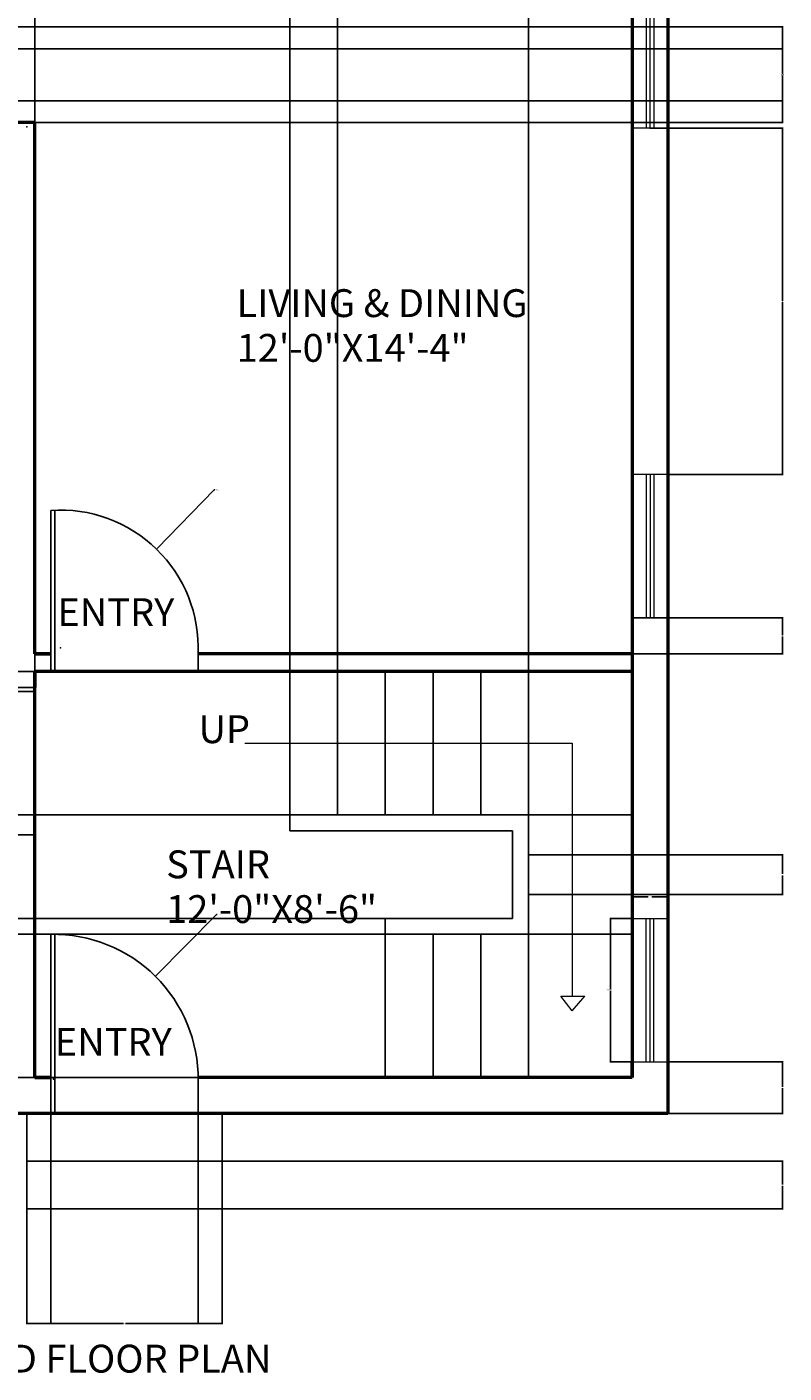
# Model space of a CAD drawing. Units: inches. Extents: x 2750 to 3097, y 1429 to 2028.
# Tile 2 of 4: x 2907 to 3097, y 1429 to 1768. Entities that reach past the tile are written whole.
import ezdxf

# ---------------------------------------------------------------- set-up
doc = ezdxf.new("R2010")
doc.units = ezdxf.units.IN
for name, color, linetype, lineweight in [('A-ANNO-DIMS', 2, 'Continuous', 18), ('A-ANNO-SYMB', 7, 'Continuous', 18), ('A-ANNO-TEXT', 7, 'Continuous', 25), ('A-AREA-IDEN', 7, 'Continuous', 25), ('A-DOOR', 3, 'Continuous', 25), ('A-FLOR-STRS', 7, 'Continuous', 25), ('A-GLAZ', 4, 'Continuous', 18), ('A-WALL', 7, 'Continuous', 50)]:
    doc.layers.add(name, color=color, linetype=linetype, lineweight=lineweight)
doc.styles.get("Standard").update_dxf_attribs({"font": 'arial.ttf'})
doc.dimstyles.get("Standard").update_dxf_attribs({"dimtxt": 0.18, "dimasz": 0.18, "dimexe": 0.18, "dimexo": 0.0625, "dimgap": 0.09, "dimtad": 0, "dimtih": 1, "dimtoh": 1, "dimdec": 4, "dimzin": 0, "dimdsep": 46, "dimtxsty": 'Standard', "dimcen": 0.09, "dimadec": 0, "dimazin": 0, "dimtfac": 1, "dimtdec": 4, "dimtofl": 0, "dimtmove": 0, "dimatfit": 3, "dimfxl": 1, "dimtolj": 1, "dimtzin": 0, "dimarcsym": 0})

# ---------------------------------------------------------------- blocks, each defined once
blk = doc.blocks.new('WIN-36IN')
for p, q in [((9, 36), (0, 36)), ((3.5, 36), (3.5, 0)), ((4.5, 36), (4.5, 0)), ((5.5, 36), (5.5, 0)), ((9, 0), (0, 0))]:
    blk.add_line(p, q)
blk = doc.blocks.new('*D7')
at = {"layer": 'A-ANNO-DIMS', "color": 0, "lineweight": -2, "transparency": 16777216}
for p, q in [((3058.46, 1543.59), (3052.94, 1543.59)), ((3053.12, 1543.41), (3053.12, 1525.78)), ((3053.12, 1507.77), (3053.12, 1525.41)), ((3058.46, 1507.59), (3052.94, 1507.59))]:
    blk.add_line(p, q, dxfattribs=at)
at = {"layer": 'A-ANNO-DIMS', "color": 0, "transparency": 16777216}
for points in [[(3053.09, 1543.41), (3053.15, 1543.41), (3053.12, 1543.59)], [(3053.09, 1507.77), (3053.15, 1507.77), (3053.12, 1507.59)]]:
    blk.add_solid(points, dxfattribs=at)
at = {"layer": 'Defpoints', "color": 0, "transparency": 16777216}
for p in [(3058.52, 1543.59), (3053.12, 1507.59), (3058.52, 1507.59)]:
    blk.add_point(p, dxfattribs=at)
at = {"layer": 'A-ANNO-DIMS', "color": 0, "transparency": 16777216, "insert": (3053.12, 1525.59), "char_height": 0.18, "attachment_point": 5}
blk.add_mtext('\\A1;WINDOW 36 TYP.', dxfattribs=at)
blk = doc.blocks.new('*D8')
at = {"layer": 'A-ANNO-DIMS', "color": 0, "lineweight": -2, "transparency": 16777216}
for p, q in [((3058.52, 1543.66), (3058.52, 1549.17)), ((3058.7, 1548.99), (3062.56, 1548.99)), ((3067.34, 1548.99), (3063.48, 1548.99)), ((3067.52, 1543.66), (3067.52, 1549.17))]:
    blk.add_line(p, q, dxfattribs=at)
at = {"layer": 'A-ANNO-DIMS', "color": 0, "transparency": 16777216}
for points in [[(3058.7, 1549.02), (3058.7, 1548.96), (3058.52, 1548.99)], [(3067.34, 1549.02), (3067.34, 1548.96), (3067.52, 1548.99)]]:
    blk.add_solid(points, dxfattribs=at)
at = {"layer": 'Defpoints', "color": 0, "transparency": 16777216}
for p in [(3058.52, 1548.99), (3058.52, 1543.59), (3067.52, 1543.59)]:
    blk.add_point(p, dxfattribs=at)
at = {"layer": 'A-ANNO-DIMS', "color": 0, "transparency": 16777216, "insert": (3063.02, 1548.99), "char_height": 0.18, "attachment_point": 5}
blk.add_mtext('\\A1;9 TYP.', dxfattribs=at)
blk = doc.blocks.new('*D16')
at = {"layer": 'A-ANNO-DIMS', "color": 0, "lineweight": -2, "transparency": 16777216}
for p, q in [((2906.52, 1470.53), (2906.52, 1441.61)), ((2955.52, 1470.53), (2955.52, 1441.61)), ((2906.7, 1441.79), (2930.8, 1441.79)), ((2955.34, 1441.79), (2931.24, 1441.79))]:
    blk.add_line(p, q, dxfattribs=at)
at = {"layer": 'A-ANNO-DIMS', "color": 0, "transparency": 16777216}
for points in [[(2906.7, 1441.82), (2906.7, 1441.76), (2906.52, 1441.79)], [(2955.34, 1441.82), (2955.34, 1441.76), (2955.52, 1441.79)]]:
    blk.add_solid(points, dxfattribs=at)
at = {"layer": 'Defpoints', "color": 0, "transparency": 16777216}
for p in [(2906.52, 1470.59), (2955.52, 1470.59), (2955.52, 1441.79)]:
    blk.add_point(p, dxfattribs=at)
at = {"layer": 'A-ANNO-DIMS', "color": 0, "transparency": 16777216, "insert": (2931.02, 1441.79), "char_height": 0.18, "attachment_point": 5}
blk.add_mtext('\\A1;49', dxfattribs=at)
blk = doc.blocks.new('*D19')
at = {"layer": 'A-ANNO-DIMS', "color": 0, "lineweight": -2, "transparency": 16777216}
for p, q in [((2912.52, 1494.53), (2912.52, 1441.61)), ((2949.52, 1494.53), (2949.52, 1441.61)), ((2912.7, 1441.79), (2930.8, 1441.79)), ((2949.34, 1441.79), (2931.24, 1441.79))]:
    blk.add_line(p, q, dxfattribs=at)
at = {"layer": 'A-ANNO-DIMS', "color": 0, "transparency": 16777216}
for points in [[(2912.7, 1441.82), (2912.7, 1441.76), (2912.52, 1441.79)], [(2949.34, 1441.82), (2949.34, 1441.76), (2949.52, 1441.79)]]:
    blk.add_solid(points, dxfattribs=at)
at = {"layer": 'Defpoints', "color": 0, "transparency": 16777216}
for p in [(2912.52, 1494.59), (2949.52, 1494.59), (2949.52, 1441.79)]:
    blk.add_point(p, dxfattribs=at)
at = {"layer": 'A-ANNO-DIMS', "color": 0, "transparency": 16777216, "insert": (2931.02, 1441.79), "char_height": 0.18, "attachment_point": 5}
blk.add_mtext('\\A1;37', dxfattribs=at)
blk = doc.blocks.new('*D24')
at = {"layer": 'A-ANNO-DIMS', "color": 0, "lineweight": -2, "transparency": 16777216}
for p, q in [((3067.58, 1507.59), (3096.5, 1507.59)), ((3096.32, 1507.41), (3096.32, 1501.27)), ((3096.32, 1494.77), (3096.32, 1500.91)), ((3067.58, 1494.59), (3096.5, 1494.59))]:
    blk.add_line(p, q, dxfattribs=at)
at = {"layer": 'A-ANNO-DIMS', "color": 0, "transparency": 16777216}
for points in [[(3096.29, 1507.41), (3096.35, 1507.41), (3096.32, 1507.59)], [(3096.29, 1494.77), (3096.35, 1494.77), (3096.32, 1494.59)]]:
    blk.add_solid(points, dxfattribs=at)
at = {"layer": 'Defpoints', "color": 0, "transparency": 16777216}
for p in [(3067.52, 1507.59), (3096.32, 1507.59), (3067.52, 1494.59)]:
    blk.add_point(p, dxfattribs=at)
at = {"layer": 'A-ANNO-DIMS', "color": 0, "transparency": 16777216, "insert": (3096.32, 1501.09), "char_height": 0.18, "attachment_point": 5}
blk.add_mtext('\\A1;13', dxfattribs=at)
blk = doc.blocks.new('*D25')
at = {"layer": 'A-ANNO-DIMS', "color": 0, "lineweight": -2, "transparency": 16777216}
for p, q in [((3058.58, 1619.09), (3096.5, 1619.09)), ((3096.32, 1618.91), (3096.32, 1614.77)), ((3096.32, 1610.27), (3096.32, 1614.41)), ((3058.58, 1610.09), (3096.5, 1610.09))]:
    blk.add_line(p, q, dxfattribs=at)
at = {"layer": 'A-ANNO-DIMS', "color": 0, "transparency": 16777216}
for points in [[(3096.29, 1618.91), (3096.35, 1618.91), (3096.32, 1619.09)], [(3096.29, 1610.27), (3096.35, 1610.27), (3096.32, 1610.09)]]:
    blk.add_solid(points, dxfattribs=at)
at = {"layer": 'Defpoints', "color": 0, "transparency": 16777216}
for p in [(3058.52, 1619.09), (3096.32, 1619.09), (3058.52, 1610.09)]:
    blk.add_point(p, dxfattribs=at)
at = {"layer": 'A-ANNO-DIMS', "color": 0, "transparency": 16777216, "insert": (3096.32, 1614.59), "char_height": 0.18, "attachment_point": 5}
blk.add_mtext('\\A1;9', dxfattribs=at)
blk = doc.blocks.new('*D26')
at = {"layer": 'A-ANNO-DIMS', "color": 0, "lineweight": -2, "transparency": 16777216}
for p, q in [((3067.58, 1742.09), (3096.5, 1742.09)), ((3096.32, 1741.91), (3096.32, 1698.77)), ((3096.32, 1655.27), (3096.32, 1698.41)), ((3067.58, 1655.09), (3096.5, 1655.09))]:
    blk.add_line(p, q, dxfattribs=at)
at = {"layer": 'A-ANNO-DIMS', "color": 0, "transparency": 16777216}
for points in [[(3096.29, 1741.91), (3096.35, 1741.91), (3096.32, 1742.09)], [(3096.29, 1655.27), (3096.35, 1655.27), (3096.32, 1655.09)]]:
    blk.add_solid(points, dxfattribs=at)
at = {"layer": 'Defpoints', "color": 0, "transparency": 16777216}
for p in [(3067.52, 1742.09), (3096.32, 1742.09), (3067.52, 1655.09)]:
    blk.add_point(p, dxfattribs=at)
at = {"layer": 'A-ANNO-DIMS', "color": 0, "transparency": 16777216, "insert": (3096.32, 1698.59), "char_height": 0.18, "attachment_point": 5}
blk.add_mtext('\\A1;87', dxfattribs=at)
blk = doc.blocks.new('*D39')
at = {"layer": 'A-ANNO-DIMS', "color": 0, "lineweight": -2, "transparency": 16777216}
for p, q in [((2860.58, 1767.56), (3096.5, 1767.56)), ((3096.32, 1767.38), (3096.32, 1755.76)), ((3096.32, 1743.77), (3096.32, 1755.4)), ((2860.58, 1743.59), (3096.5, 1743.59))]:
    blk.add_line(p, q, dxfattribs=at)
at = {"layer": 'A-ANNO-DIMS', "color": 0, "transparency": 16777216}
for points in [[(3096.29, 1767.38), (3096.35, 1767.38), (3096.32, 1767.56)], [(3096.29, 1743.77), (3096.35, 1743.77), (3096.32, 1743.59)]]:
    blk.add_solid(points, dxfattribs=at)
at = {"layer": 'Defpoints', "color": 0, "transparency": 16777216}
for p in [(2860.52, 1767.56), (3096.32, 1767.56), (2860.52, 1743.59)]:
    blk.add_point(p, dxfattribs=at)
at = {"layer": 'A-ANNO-DIMS', "color": 0, "transparency": 16777216, "insert": (3096.32, 1755.58), "char_height": 0.18, "attachment_point": 5}
blk.add_mtext('\\A1;23.97', dxfattribs=at)
blk = doc.blocks.new('*D48')
at = {"layer": 'A-ANNO-DIMS', "color": 0, "lineweight": -2, "transparency": 16777216}
for p, q in [((2853.77, 1762.1), (3096.5, 1762.1)), ((3096.32, 1761.92), (3096.32, 1755.71)), ((3096.32, 1749.14), (3096.32, 1755.35)), ((2853.77, 1748.96), (3096.5, 1748.96))]:
    blk.add_line(p, q, dxfattribs=at)
at = {"layer": 'A-ANNO-DIMS', "color": 0, "transparency": 16777216}
for points in [[(3096.29, 1761.92), (3096.35, 1761.92), (3096.32, 1762.1)], [(3096.29, 1749.14), (3096.35, 1749.14), (3096.32, 1748.96)]]:
    blk.add_solid(points, dxfattribs=at)
at = {"layer": 'Defpoints', "color": 0, "transparency": 16777216}
for p in [(2853.71, 1762.1), (3096.32, 1762.1), (2853.71, 1748.96)]:
    blk.add_point(p, dxfattribs=at)
at = {"layer": 'A-ANNO-DIMS', "color": 0, "transparency": 16777216, "insert": (3096.32, 1755.53), "char_height": 0.18, "attachment_point": 5}
blk.add_mtext('\\A1;13.143', dxfattribs=at)
blk = doc.blocks.new('*D51')
at = {"layer": 'A-ANNO-DIMS', "color": 0, "lineweight": -2, "transparency": 16777216}
for p, q in [((2972.52, 1605.66), (2972.52, 2027.57)), ((2972.7, 2027.39), (2978.31, 2027.39)), ((2984.34, 2027.39), (2978.73, 2027.39)), ((2984.52, 1605.66), (2984.52, 2027.57))]:
    blk.add_line(p, q, dxfattribs=at)
at = {"layer": 'A-ANNO-DIMS', "color": 0, "transparency": 16777216}
for points in [[(2972.7, 2027.42), (2972.7, 2027.36), (2972.52, 2027.39)], [(2984.34, 2027.42), (2984.34, 2027.36), (2984.52, 2027.39)]]:
    blk.add_solid(points, dxfattribs=at)
at = {"layer": 'Defpoints', "color": 0, "transparency": 16777216}
for p in [(2984.52, 2027.39), (2972.52, 1605.59), (2984.52, 1605.59)]:
    blk.add_point(p, dxfattribs=at)
at = {"layer": 'A-ANNO-DIMS', "color": 0, "transparency": 16777216, "insert": (2978.52, 2027.39), "char_height": 0.18, "attachment_point": 5}
blk.add_mtext('\\A1;12', dxfattribs=at)
blk = doc.blocks.new('*D52')
at = {"layer": 'A-ANNO-DIMS', "color": 0, "lineweight": -2, "transparency": 16777216}
for p, q in [((2908.52, 1605.66), (2908.52, 2027.57)), ((2908.7, 2027.39), (2940.3, 2027.39)), ((2972.34, 2027.39), (2940.74, 2027.39)), ((2972.52, 1605.66), (2972.52, 2027.57))]:
    blk.add_line(p, q, dxfattribs=at)
at = {"layer": 'A-ANNO-DIMS', "color": 0, "transparency": 16777216}
for points in [[(2908.7, 2027.42), (2908.7, 2027.36), (2908.52, 2027.39)], [(2972.34, 2027.42), (2972.34, 2027.36), (2972.52, 2027.39)]]:
    blk.add_solid(points, dxfattribs=at)
at = {"layer": 'Defpoints', "color": 0, "transparency": 16777216}
for p in [(2972.52, 2027.39), (2908.52, 1605.59), (2972.52, 1605.59)]:
    blk.add_point(p, dxfattribs=at)
at = {"layer": 'A-ANNO-DIMS', "color": 0, "transparency": 16777216, "insert": (2940.52, 2027.39), "char_height": 0.18, "attachment_point": 5}
blk.add_mtext('\\A1;64', dxfattribs=at)
blk = doc.blocks.new('*D53')
at = {"layer": 'A-ANNO-DIMS', "color": 0, "lineweight": -2, "transparency": 16777216}
for p, q in [((3032.52, 1605.66), (3032.52, 2027.57)), ((3032.7, 2027.39), (3045.3, 2027.39)), ((3058.34, 2027.39), (3045.74, 2027.39)), ((3058.52, 1605.66), (3058.52, 2027.57))]:
    blk.add_line(p, q, dxfattribs=at)
at = {"layer": 'A-ANNO-DIMS', "color": 0, "transparency": 16777216}
for points in [[(3032.7, 2027.42), (3032.7, 2027.36), (3032.52, 2027.39)], [(3058.34, 2027.42), (3058.34, 2027.36), (3058.52, 2027.39)]]:
    blk.add_solid(points, dxfattribs=at)
at = {"layer": 'Defpoints', "color": 0, "transparency": 16777216}
for p in [(3058.52, 2027.39), (3032.52, 1605.59), (3058.52, 1605.59)]:
    blk.add_point(p, dxfattribs=at)
at = {"layer": 'A-ANNO-DIMS', "color": 0, "transparency": 16777216, "insert": (3045.52, 2027.39), "char_height": 0.18, "attachment_point": 5}
blk.add_mtext('\\A1;26', dxfattribs=at)
blk = doc.blocks.new('*D54')
at = {"layer": 'A-ANNO-DIMS', "color": 0, "lineweight": -2, "transparency": 16777216}
for p, q in [((2972.46, 1605.59), (2750.54, 1605.59)), ((2750.72, 1605.41), (2750.72, 1587.77)), ((2750.72, 1569.77), (2750.72, 1587.41)), ((2972.46, 1569.59), (2750.54, 1569.59))]:
    blk.add_line(p, q, dxfattribs=at)
at = {"layer": 'A-ANNO-DIMS', "color": 0, "transparency": 16777216}
for points in [[(2750.69, 1605.41), (2750.75, 1605.41), (2750.72, 1605.59)], [(2750.69, 1569.77), (2750.75, 1569.77), (2750.72, 1569.59)]]:
    blk.add_solid(points, dxfattribs=at)
at = {"layer": 'Defpoints', "color": 0, "transparency": 16777216}
for p in [(2750.72, 1605.59), (2972.52, 1605.59), (2972.52, 1569.59)]:
    blk.add_point(p, dxfattribs=at)
at = {"layer": 'A-ANNO-DIMS', "color": 0, "transparency": 16777216, "insert": (2750.72, 1587.59), "char_height": 0.18, "attachment_point": 5}
blk.add_mtext('\\A1;36', dxfattribs=at)
blk = doc.blocks.new('*D55')
at = {"layer": 'A-ANNO-DIMS', "color": 0, "lineweight": -2, "transparency": 16777216}
for p, q in [((3058.58, 1559.59), (3096.5, 1559.59)), ((3096.32, 1559.41), (3096.32, 1554.77)), ((3096.32, 1549.77), (3096.32, 1554.41)), ((3058.58, 1549.59), (3096.5, 1549.59))]:
    blk.add_line(p, q, dxfattribs=at)
at = {"layer": 'A-ANNO-DIMS', "color": 0, "transparency": 16777216}
for points in [[(3096.29, 1559.41), (3096.35, 1559.41), (3096.32, 1559.59)], [(3096.29, 1549.77), (3096.35, 1549.77), (3096.32, 1549.59)]]:
    blk.add_solid(points, dxfattribs=at)
at = {"layer": 'Defpoints', "color": 0, "transparency": 16777216}
for p in [(3058.52, 1559.59), (3096.32, 1559.59), (3058.52, 1549.59)]:
    blk.add_point(p, dxfattribs=at)
at = {"layer": 'A-ANNO-DIMS', "color": 0, "transparency": 16777216, "insert": (3096.32, 1554.59), "char_height": 0.18, "attachment_point": 5}
blk.add_mtext('\\A1;10', dxfattribs=at)
blk = doc.blocks.new('*D56')
at = {"layer": 'A-ANNO-DIMS', "color": 0, "lineweight": -2, "transparency": 16777216}
for p, q in [((2996.46, 1539.59), (2750.54, 1539.59)), ((2750.72, 1539.41), (2750.72, 1521.77)), ((2750.72, 1503.77), (2750.72, 1521.41)), ((2996.46, 1503.59), (2750.54, 1503.59))]:
    blk.add_line(p, q, dxfattribs=at)
at = {"layer": 'A-ANNO-DIMS', "color": 0, "transparency": 16777216}
for points in [[(2750.69, 1539.41), (2750.75, 1539.41), (2750.72, 1539.59)], [(2750.69, 1503.77), (2750.75, 1503.77), (2750.72, 1503.59)]]:
    blk.add_solid(points, dxfattribs=at)
at = {"layer": 'Defpoints', "color": 0, "transparency": 16777216}
for p in [(2750.72, 1539.59), (2996.52, 1539.59), (2996.52, 1503.59)]:
    blk.add_point(p, dxfattribs=at)
at = {"layer": 'A-ANNO-DIMS', "color": 0, "transparency": 16777216, "insert": (2750.72, 1521.59), "char_height": 0.18, "attachment_point": 5}
blk.add_mtext('\\A1;36', dxfattribs=at)
blk = doc.blocks.new('*D57')
at = {"layer": 'A-ANNO-DIMS', "color": 0, "lineweight": -2, "transparency": 16777216}
for p, q in [((2996.457604, 1543.592536), (2750.540104, 1543.592536)), ((2750.720104, 1543.412536), (2750.720104, 1541.772536)), ((2996.457604, 1539.592536), (2750.540104, 1539.592536)), ((2750.720104, 1539.772536), (2750.720104, 1541.412536))]:
    blk.add_line(p, q, dxfattribs=at)
at = {"layer": 'A-ANNO-DIMS', "color": 0, "transparency": 16777216}
for points in [[(2750.690104, 1543.412536), (2750.750104, 1543.412536), (2750.720104, 1543.592536)], [(2750.690104, 1539.772536), (2750.750104, 1539.772536), (2750.720104, 1539.592536)]]:
    blk.add_solid(points, dxfattribs=at)
at = {"layer": 'Defpoints', "color": 0, "transparency": 16777216}
for p in [(2750.720104, 1543.592536), (2996.520104, 1543.592536), (2996.520104, 1539.592536)]:
    blk.add_point(p, dxfattribs=at)
at = {"layer": 'A-ANNO-DIMS', "color": 0, "transparency": 16777216, "insert": (2750.720104, 1541.592536), "char_height": 0.18, "attachment_point": 5}
blk.add_mtext('\\A1;4', dxfattribs=at)
blk = doc.blocks.new('*D58')
at = {"layer": 'A-ANNO-DIMS', "color": 0, "lineweight": -2, "transparency": 16777216}
for p, q in [((2955.58, 1482.59), (3096.5, 1482.59)), ((3096.32, 1482.41), (3096.32, 1476.77)), ((3096.32, 1470.77), (3096.32, 1476.41)), ((2955.58, 1470.59), (3096.5, 1470.59))]:
    blk.add_line(p, q, dxfattribs=at)
at = {"layer": 'A-ANNO-DIMS', "color": 0, "transparency": 16777216}
for points in [[(3096.29, 1482.41), (3096.35, 1482.41), (3096.32, 1482.59)], [(3096.29, 1470.77), (3096.35, 1470.77), (3096.32, 1470.59)]]:
    blk.add_solid(points, dxfattribs=at)
at = {"layer": 'Defpoints', "color": 0, "transparency": 16777216}
for p in [(2955.52, 1482.59), (3096.32, 1482.59), (2955.52, 1470.59)]:
    blk.add_point(p, dxfattribs=at)
at = {"layer": 'A-ANNO-DIMS', "color": 0, "transparency": 16777216, "insert": (3096.32, 1476.59), "char_height": 0.18, "attachment_point": 5}
blk.add_mtext('\\A1;12', dxfattribs=at)
blk = doc.blocks.new('*D61')
at = {"layer": 'A-ANNO-DIMS', "color": 0, "lineweight": -2, "transparency": 16777216}
for p, q in [((2906.38, 1742.43), (2906.56, 1742.43)), ((2906.47, 1742.34), (2906.47, 1742.52)), ((2861.05, 1698.28), (2877.95, 1714.71)), ((2860.87, 1698.28), (2861.05, 1698.28))]:
    blk.add_line(p, q, dxfattribs=at)
at = {"layer": 'A-ANNO-DIMS', "color": 0, "transparency": 16777216}
blk.add_solid([(2877.93, 1714.73), (2877.98, 1714.69), (2878.08, 1714.83)], dxfattribs=at)
at = {"layer": 'Defpoints', "color": 0, "transparency": 16777216}
for p in [(2906.47, 1742.43), (2878.08, 1714.83)]:
    blk.add_point(p, dxfattribs=at)
at = {"layer": 'A-ANNO-DIMS', "color": 0, "transparency": 16777216, "insert": (2860.39, 1698.28), "char_height": 0.18, "attachment_point": 5}
blk.add_mtext('\\A1;R39.59', dxfattribs=at)
blk = doc.blocks.new('*D62')
at = {"layer": 'A-ANNO-DIMS', "color": 0, "lineweight": -2, "transparency": 16777216}
for p, q in [((2954.13, 1544.54), (2938.9, 1529.18)), ((2954.31, 1544.54), (2954.13, 1544.54)), ((2913.08, 1503.24), (2913.26, 1503.24)), ((2913.17, 1503.15), (2913.17, 1503.33))]:
    blk.add_line(p, q, dxfattribs=at)
at = {"layer": 'A-ANNO-DIMS', "color": 0, "transparency": 16777216}
blk.add_solid([(2938.87, 1529.2), (2938.92, 1529.16), (2938.77, 1529.06)], dxfattribs=at)
at = {"layer": 'Defpoints', "color": 0, "transparency": 16777216}
for p in [(2938.77, 1529.06), (2913.17, 1503.24)]:
    blk.add_point(p, dxfattribs=at)
at = {"layer": 'A-ANNO-DIMS', "color": 0, "transparency": 16777216, "insert": (2954.86, 1544.54), "char_height": 0.18, "attachment_point": 5}
blk.add_mtext('\\A1;R36.355', dxfattribs=at)
blk = doc.blocks.new('*D64')
at = {"layer": 'A-ANNO-DIMS', "color": 0, "lineweight": -2, "transparency": 16777216}
for p, q in [((2953.56, 1651.26), (2939.2, 1636.5)), ((2953.74, 1651.26), (2953.56, 1651.26)), ((2914.85, 1611.56), (2915.03, 1611.56)), ((2914.94, 1611.47), (2914.94, 1611.65))]:
    blk.add_line(p, q, dxfattribs=at)
at = {"layer": 'A-ANNO-DIMS', "color": 0, "transparency": 16777216}
blk.add_solid([(2939.18, 1636.52), (2939.22, 1636.48), (2939.08, 1636.37)], dxfattribs=at)
at = {"layer": 'Defpoints', "color": 0, "transparency": 16777216}
for p in [(2939.08, 1636.37), (2914.94, 1611.56)]:
    blk.add_point(p, dxfattribs=at)
at = {"layer": 'A-ANNO-DIMS', "color": 0, "transparency": 16777216, "insert": (2954.2, 1651.26), "char_height": 0.18, "attachment_point": 5}
blk.add_mtext('\\A1;R34.61', dxfattribs=at)

msp = doc.modelspace()

# ---------------------------------------------------------------- linework, layer by layer
at = {"layer": 'A-ANNO-SYMB'}
for p, q in [((2961.2831, 1587.6242), (3043.4359, 1587.6242)), ((3043.4359, 1587.6242), (3043.4359, 1524.1416)), ((3040.6197, 1524.0478), (3046.6197, 1524.0478)), ((3043.4359, 1520.367), (3040.6197, 1524.0478)), ((3043.4359, 1524.1416), (3043.4359, 1524.0478)), ((3043.4359, 1520.367), (3046.6197, 1524.0478))]:
    msp.add_line(p, q, dxfattribs=at)
at = {"layer": 'A-DOOR'}
for p, q in [((2912.5201, 1610.0927), (2912.5201, 1646.0927)), ((2913.5201, 1610.0927), (2913.5201, 1646.0927)), ((2912.5201, 1610.0927), (2912.5201, 1605.5925)), ((2913.5201, 1610.0927), (2913.5201, 1605.5925)), ((2949.5201, 1605.5925), (2949.5201, 1610.0925)), ((2913.5201, 1605.5925), (2949.5201, 1605.5925)), ((2908.534, 1601.5926), (2904.0201, 1601.5926)), ((2904.0201, 1600.5926), (2908.5201, 1600.5926)), ((2908.5201, 1600.5926), (2908.5201, 1564.5926)), ((2908.5201, 1564.5926), (2904.0201, 1564.5926)), ((2912.5201, 1503.5925), (2912.5201, 1539.5925)), ((2913.5201, 1503.5925), (2913.5201, 1539.5925)), ((2912.5201, 1503.5925), (2912.5201, 1494.5925)), ((2913.5201, 1503.5925), (2913.5201, 1494.5925)), ((2949.5201, 1494.5925), (2949.5201, 1503.5925)), ((2913.5201, 1494.5925), (2949.5201, 1494.5925))]:
    msp.add_line(p, q, dxfattribs=at)
for centre, radius, start, end in [((2914.9379, 1611.5638), 34.6134, 357.563902, 94.005512), ((2913.167, 1503.2435), 36.3547, 359.449976, 91.019625)]:
    msp.add_arc(centre, radius, start, end, dxfattribs=at)
at = {"layer": 'A-FLOR-STRS'}
for p, q in [((2972.5201, 1605.5925), (2972.5201, 1565.5925)), ((2972.5201, 1605.5925), (2995.5201, 1605.5925)), ((2972.5201, 1605.5925), (2984.5201, 1605.5925)), ((2984.5201, 1605.5925), (2984.5201, 1569.5925)), ((2996.5201, 1569.5925), (2996.5201, 1605.5925)), ((2996.5201, 1605.5925), (2996.5201, 1569.5925)), ((3008.5201, 1569.5925), (3008.5201, 1605.5925)), ((3008.5201, 1605.5925), (3008.5201, 1569.5925)), ((3020.5201, 1569.5925), (3020.5201, 1605.5925)), ((3032.5201, 1569.5925), (3032.5201, 1605.5925)), ((3032.5201, 1605.5925), (3032.5201, 1569.5925)), ((2984.5201, 1569.5925), (2972.5201, 1569.5925)), ((2984.5201, 1569.5925), (2996.5201, 1569.5925)), ((2996.5201, 1569.5925), (3008.5201, 1569.5925)), ((3008.5201, 1569.5925), (3020.5201, 1569.5925)), ((3020.5201, 1569.5925), (3032.5201, 1569.5925)), ((3032.5201, 1569.5925), (3032.5201, 1503.5925)), ((3032.5201, 1569.5925), (3058.5201, 1569.5925)), ((3032.5201, 1569.5925), (3032.5201, 1559.5925)), ((2984.5201, 1565.5925), (2972.5201, 1565.5925)), ((2984.5201, 1565.5925), (2996.5201, 1565.5925)), ((2996.5201, 1565.5925), (3008.5201, 1565.5925)), ((3008.5201, 1565.5925), (3020.5201, 1565.5925)), ((3020.5201, 1565.5925), (3028.5201, 1565.5925)), ((3028.5201, 1565.5925), (3028.5201, 1543.5925)), ((3032.5201, 1559.5925), (3058.5201, 1559.5925)), ((3032.5201, 1559.5925), (3032.5201, 1549.5925)), ((3032.5201, 1549.5925), (3058.5201, 1549.5925)), ((3008.5201, 1543.5925), (2996.5201, 1543.5925)), ((2996.5201, 1543.5925), (2996.5201, 1539.5925)), ((3020.5201, 1543.5925), (3008.5201, 1543.5925)), ((3020.5201, 1543.5925), (3028.5201, 1543.5925)), ((3008.5201, 1539.5925), (2996.5201, 1539.5925)), ((2996.5201, 1539.5925), (2996.5201, 1503.5925)), ((3020.5201, 1539.5925), (3008.5201, 1539.5925)), ((3008.5201, 1539.5925), (3008.5201, 1503.5925)), ((3020.5201, 1503.5925), (3020.5201, 1539.5925)), ((3020.5201, 1539.5925), (3032.5201, 1539.5925)), ((3032.5201, 1539.5925), (3058.5201, 1539.5925)), ((3032.5201, 1503.5925), (3020.5201, 1503.5925)), ((2912.5201, 1494.5925), (2906.5201, 1494.5925)), ((2906.5201, 1494.5925), (2906.5201, 1482.5925)), ((2949.5201, 1494.5925), (2955.5201, 1494.5925)), ((2955.5201, 1494.5925), (2955.5201, 1482.5925)), ((2955.5201, 1482.5925), (2906.5201, 1482.5925)), ((2906.5201, 1482.5925), (2906.5201, 1470.5925)), ((2955.5201, 1482.5925), (2955.5201, 1470.5925)), ((2955.5201, 1470.5925), (2906.5201, 1470.5925))]:
    msp.add_line(p, q, dxfattribs=at)
at = {"layer": 'A-GLAZ'}
for p, q in [((3062.0172, 1778.0925), (3062.0172, 1742.0925)), ((3063.0172, 1778.0925), (3063.0172, 1742.0925)), ((3064.0172, 1778.0925), (3064.0172, 1742.0925)), ((3067.5201, 1742.0925), (3058.5201, 1742.0925)), ((3063.0172, 1742.0925), (3067.5201, 1742.0925)), ((3063.0201, 1655.0925), (3058.5201, 1655.0925)), ((3063.0201, 1619.0925), (3067.5201, 1619.0925)), ((3063.0201, 1543.5925), (3067.5201, 1543.5925))]:
    msp.add_line(p, q, dxfattribs=at)
at = {"layer": 'A-WALL'}
for p, q in [((3067.5201, 1998.5925), (3067.5201, 1494.5925)), ((3058.5201, 1989.5925), (3058.5201, 1503.5925)), ((2788.5201, 1743.5925), (2908.5201, 1743.5925)), ((2908.5201, 1610.0925), (2908.5201, 1743.5925)), ((2908.5201, 1610.0925), (2912.5201, 1610.0927)), ((2912.5201, 1610.0925), (2908.5201, 1610.0925)), ((3058.5201, 1610.0925), (2949.5201, 1610.0925)), ((3058.5201, 1605.5925), (2908.5201, 1605.5925)), ((2908.5201, 1503.5925), (2908.5201, 1605.5925)), ((2908.5201, 1605.5925), (2908.534, 1601.5926)), ((3058.5201, 1503.5925), (3058.5201, 1507.5925)), ((2908.5201, 1503.5925), (2912.5201, 1503.5925)), ((2912.5201, 1503.5925), (2908.5201, 1503.5925)), ((3058.5201, 1503.5925), (2949.5201, 1503.5925)), ((3067.5201, 1494.5925), (2779.5201, 1494.5925))]:
    msp.add_line(p, q, dxfattribs=at)

# ---------------------------------------------------------------- block references
at = {"layer": 'A-GLAZ'}
msp.add_blockref('WIN-36IN', (3058.52, 1619.093), dxfattribs=at)
at = {"layer": 'A-GLAZ', "rotation": 180}
msp.add_blockref('WIN-36IN', (3067.5202, 1543.5921), dxfattribs=at)

# ---------------------------------------------------------------- texts
at = {"layer": 'A-ANNO-TEXT'}
for s, p in [('ENTRY', (2914.1726, 1617.0275)), ('UP', (2949.6283, 1587.6242)), ('ENTRY', (2913.5201, 1509.0671)), ('GROUND FLOOR PLAN', (2868.9383, 1429.4831))]:
    msp.add_text(s, height=7, dxfattribs=at).set_placement(p)
at = {"layer": 'A-AREA-IDEN'}
for s, p in [('LIVING & DINING', (2959.1858, 1694.6677)), ('12\'-0"X14\'-4"', (2959.1858, 1683.4228)), ('STAIR', (2941.4928, 1553.6738)), ('12\'-0"X8\'-6"', (2941.4928, 1542.4289))]:
    msp.add_text(s, height=7, dxfattribs=at).set_placement(p)

# ---------------------------------------------------------------- dimensions: what is measured, and where the dimension line sits
at = {"layer": 'A-ANNO-DIMS'}
for base, p1, p2, picture, middle in [((2972.5201, 2027.3925), (2908.5201, 1605.5925), (2972.5201, 1605.5925), '*D52', (2940.5201, 2027.3925)), ((2984.5201, 2027.3925), (2972.5201, 1605.5925), (2984.5201, 1605.5925), '*D51', (2978.5201, 2027.3925)), ((3058.5201, 2027.3925), (3032.5201, 1605.5925), (3058.5201, 1605.5925), '*D53', (3045.5201, 2027.3925)), ((2949.5201, 1441.7925), (2912.5201, 1494.5925), (2949.5201, 1494.5925), '*D19', (2931.0201, 1441.7925)), ((2955.5201, 1441.7925), (2906.5201, 1470.5925), (2955.5201, 1470.5925), '*D16', (2931.0201, 1441.7925))]:
    dim = msp.add_linear_dim(base=base, p1=p1, p2=p2, dimstyle='Standard', override={"dimdec": 0, "dimlfac": 1, "dimrnd": 0, "dimzin": 0, "dimdsep": 46, "dimlunit": 2}, dxfattribs=at)
    dim.commit()
    dim.dimension.update_dxf_attribs({"geometry": picture, "text_midpoint": middle})
for base, p1, p2, override, picture, middle in [((3096.3201, 1767.5629), (2860.5201, 1743.5925), (2860.5201, 1767.5629), {"dimdec": 2, "dimlfac": 1, "dimrnd": 0, "dimzin": 0, "dimdsep": 46, "dimlunit": 2}, '*D39', (3096.3201, 1755.5777)), ((3096.3201, 1762.1022), (2853.7089, 1748.9592), (2853.7089, 1762.1022), {"dimdec": 3, "dimlfac": 1, "dimrnd": 0, "dimzin": 0, "dimdsep": 46, "dimlunit": 2}, '*D48', (3096.3201, 1755.5307)), ((3096.3201, 1742.0925), (3067.5201, 1655.0925), (3067.5201, 1742.0925), {"dimdec": 0, "dimlfac": 1, "dimrnd": 0, "dimzin": 0, "dimdsep": 46, "dimlunit": 2}, '*D26', (3096.3201, 1698.5925)), ((3096.3201, 1619.0925), (3058.5201, 1610.0925), (3058.5201, 1619.0925), {"dimdec": 0, "dimlfac": 1, "dimrnd": 0, "dimzin": 0, "dimdsep": 46, "dimlunit": 2}, '*D25', (3096.3201, 1614.5925)), ((2750.7201, 1605.5925), (2972.5201, 1569.5925), (2972.5201, 1605.5925), {"dimdec": 0, "dimlfac": 1, "dimrnd": 0, "dimzin": 0, "dimdsep": 46, "dimlunit": 2}, '*D54', (2750.7201, 1587.5925)), ((3096.3201, 1559.5925), (3058.5201, 1549.5925), (3058.5201, 1559.5925), {"dimdec": 0, "dimlfac": 1, "dimrnd": 0, "dimzin": 0, "dimdsep": 46, "dimlunit": 2}, '*D55', (3096.3201, 1554.5925)), ((2750.7201, 1543.5925), (2996.5201, 1539.5925), (2996.5201, 1543.5925), {"dimdec": 0, "dimlfac": 1, "dimrnd": 0, "dimzin": 0, "dimdsep": 46, "dimlunit": 2}, '*D57', (2750.7201, 1541.5925)), ((2750.7201, 1539.5925), (2996.5201, 1503.5925), (2996.5201, 1539.5925), {"dimdec": 0, "dimlfac": 1, "dimrnd": 0, "dimzin": 0, "dimdsep": 46, "dimlunit": 2}, '*D56', (2750.7201, 1521.5925)), ((3096.3201, 1507.5925), (3067.5201, 1494.5925), (3067.5201, 1507.5925), {"dimdec": 0, "dimlfac": 1, "dimrnd": 0, "dimzin": 0, "dimdsep": 46, "dimlunit": 2}, '*D24', (3096.3201, 1501.0925)), ((3096.3201, 1482.5925), (2955.5201, 1470.5925), (2955.5201, 1482.5925), {"dimdec": 0, "dimlfac": 1, "dimrnd": 0, "dimzin": 0, "dimdsep": 46, "dimlunit": 2}, '*D58', (3096.3201, 1476.5925))]:
    dim = msp.add_linear_dim(base=base, p1=p1, p2=p2, angle=90, dimstyle='Standard', override=override, dxfattribs=at)
    dim.commit()
    dim.dimension.update_dxf_attribs({"geometry": picture, "text_midpoint": middle})
for center, mpoint, override, picture, middle in [((2906.4716, 1742.4343), (2878.0839, 1714.8349), {"dimdec": 2, "dimlfac": 1, "dimrnd": 0, "dimzin": 0, "dimdsep": 46, "dimlunit": 2}, '*D61', (2860.3913, 1698.2753)), ((2914.9379, 1611.5638), (2939.076, 1636.372), {"dimdec": 2, "dimlfac": 1, "dimrnd": 0, "dimzin": 0, "dimdsep": 46, "dimlunit": 2}, '*D64', (2954.2013, 1651.2569)), ((2913.167, 1503.2435), (2938.7683, 1529.0553), {"dimdec": 3, "dimlfac": 1, "dimrnd": 0, "dimzin": 0, "dimdsep": 46, "dimlunit": 2}, '*D62', (2954.8594, 1544.5423))]:
    dim = msp.add_radius_dim(center=center, mpoint=mpoint, dimstyle='Standard', override=override, dxfattribs=at)
    dim.commit()
    dim.dimension.update_dxf_attribs({"geometry": picture, "text_midpoint": middle, "dimtype": 164})
for base, p1, p2, angle, text, picture, middle in [((3058.5201, 1548.9925), (3067.5201, 1543.5925), (3058.5201, 1543.5925), 180, '<> TYP.', '*D8', (3063.0201, 1548.9925)), ((3053.1201, 1507.5925), (3058.5201, 1543.5925), (3058.5201, 1507.5925), 270, 'WINDOW <> TYP.', '*D7', (3053.1201, 1525.5925))]:
    dim = msp.add_linear_dim(base=base, p1=p1, p2=p2, angle=angle, text=text, dimstyle='Standard', override={"dimdec": 0, "dimlfac": 1, "dimrnd": 0, "dimzin": 0, "dimdsep": 46, "dimlunit": 2}, dxfattribs=at)
    dim.commit()
    dim.dimension.update_dxf_attribs({"geometry": picture, "text_midpoint": middle})

doc.saveas('drawing.dxf')
